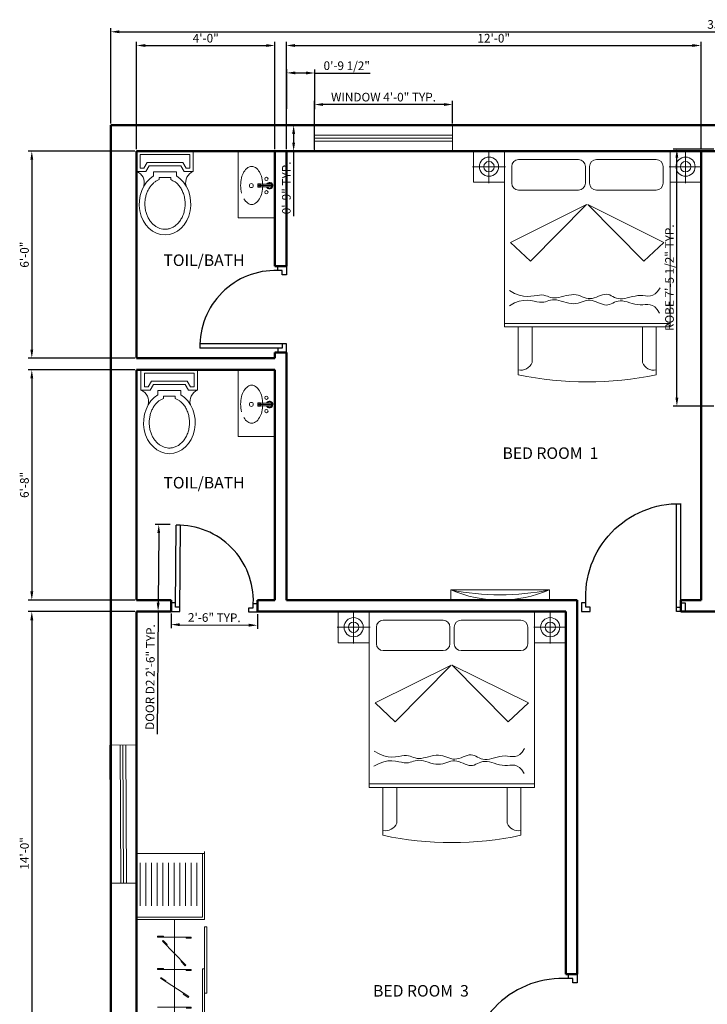
# Model space of a CAD drawing. Units: inches. Extents: x 108 to 1546, y -229 to 513.
# Tile 5 of 11: x 591 to 830, y 171 to 513. Entities that reach past the tile are written whole.
import ezdxf

# ---------------------------------------------------------------- set-up
doc = ezdxf.new("R2010")
doc.units = ezdxf.units.IN
for name, color, linetype, lineweight in [('A-ANNO-DIMS', 2, 'Continuous', 18), ('A-AREA-IDEN', 4, 'Continuous', 18), ('A-FLOR-FIXT', 9, 'Continuous', 18), ('A-FURN', 8, 'Continuous', 13), ('door', 1, 'Continuous', 25), ('tv', 2, 'Continuous', 13), ('wall', 7, 'Continuous', 50), ('WINDOW', 212, 'Continuous', 18)]:
    doc.layers.add(name, color=color, linetype=linetype, lineweight=lineweight)
doc.styles.get("Standard").update_dxf_attribs({"font": 'arial.ttf'})
doc.dimstyles.new('ISO-25', dxfattribs={"dimtxt": 3, "dimasz": 3, "dimexe": 1.25, "dimexo": 0.625, "dimtad": 1, "dimdec": 1, "dimlunit": 3, "dimtxsty": 'Standard', "dimcen": 2.5, "dimadec": 0, "dimazin": 0, "dimtfac": 1, "dimtdec": 1, "dimtmove": 0, "dimatfit": 3, "dimfxl": 1, "dimarcsym": 0})

# ---------------------------------------------------------------- blocks, each defined once
blk = doc.blocks.new('A$C4F543DC7')
for p, q in [((0.013, 3.35, -0.169), (3.313, 3.35, -0.169)), ((0.463, 3.35, -0.169), (0.013, 3.35, -0.169)), ((0.013, 2.896, -0.169), (0.013, 3.35, -0.169)), ((0.013, 3.35, -0.169), (0.013, 2.896, -0.169)), ((0.238, 3.123, -0.439), (0.238, 3.361, -0.439)), ((0.463, 3.35, -0.169), (0.463, 0.8, -0.169)), ((2.863, 3.35, -0.169), (0.463, 3.35, -0.169)), ((0.463, 2.896, -0.169), (0.463, 3.35, -0.169)), ((2.863, 0.8, -0.169), (2.863, 3.35, -0.169)), ((2.863, 3.35, -0.169), (3.313, 3.35, -0.169)), ((2.863, 2.896, -0.169), (2.863, 3.35, -0.169)), ((3.089, 3.123, -0.439), (3.089, 3.361, -0.439)), ((3.313, 3.35, -0.169), (3.313, 2.896, -0.169)), ((3.313, 3.35, -0.169), (3.313, 2.896, -0.169)), ((1.535, 3.226, -0.169), (0.668, 3.226, -0.169)), ((2.664, 3.226, -0.169), (1.797, 3.226, -0.169)), ((0.238, 3.123, -0.439), (0, 3.123, -0.439)), ((0.238, 3.123, -0.439), (0.476, 3.123, -0.439)), ((0.238, 3.123, -0.439), (0.238, 2.885, -0.439)), ((0.568, 3.126, -0.169), (0.568, 2.884, -0.169)), ((1.635, 2.884, -0.169), (1.635, 3.126, -0.169)), ((1.697, 3.126, -0.169), (1.697, 2.884, -0.169)), ((2.764, 2.884, -0.169), (2.764, 3.126, -0.169)), ((3.089, 3.123, -0.439), (2.851, 3.123, -0.439)), ((3.089, 3.123, -0.439), (3.089, 2.885, -0.439)), ((3.089, 3.123, -0.439), (3.327, 3.123, -0.439)), ((0.463, 2.896, -0.169), (0.013, 2.896, -0.169)), ((0.013, 2.896, -0.169), (0.463, 2.896, -0.169)), ((0.463, 0.8, -0.169), (0.463, 2.896, -0.169)), ((2.863, 2.896, -0.169), (2.863, 0.8, -0.169)), ((3.313, 2.896, -0.169), (2.863, 2.896, -0.169)), ((3.313, 2.896, -0.169), (2.863, 2.896, -0.169)), ((0.668, 2.784, -0.169), (1.535, 2.784, -0.169)), ((1.797, 2.784, -0.169), (2.664, 2.784, -0.169)), ((1.653, 2.573, -0.169), (0.55, 2.025, -0.169)), ((0.841, 1.752, -0.169), (1.653, 2.573, -0.169)), ((2.481, 1.752, -0.169), (1.669, 2.573, -0.169)), ((1.669, 2.573, -0.169), (2.772, 2.025, -0.169)), ((0.55, 2.025, -0.169), (0.841, 1.752, -0.169)), ((2.772, 2.025, -0.169), (2.481, 1.752, -0.169)), ((0.537, 1.327, -0.169), (0.609, 1.284, -0.169)), ((2.648, 1.277, -0.169), (2.683, 1.312, -0.169)), ((2.683, 1.312, -0.169), (2.718, 1.364, -0.169)), ((0.533, 1.105, -0.169), (0.607, 1.146, -0.169)), ((0.607, 1.146, -0.169), (0.674, 1.171, -0.169)), ((0.609, 1.284, -0.169), (0.676, 1.257, -0.169)), ((0.674, 1.171, -0.169), (0.736, 1.183, -0.169)), ((0.676, 1.257, -0.169), (0.737, 1.243, -0.169)), ((0.736, 1.183, -0.169), (0.793, 1.185, -0.169)), ((0.737, 1.243, -0.169), (0.794, 1.239, -0.169)), ((0.793, 1.185, -0.169), (0.845, 1.18, -0.169)), ((0.794, 1.239, -0.169), (0.846, 1.242, -0.169)), ((0.845, 1.18, -0.169), (0.891, 1.172, -0.169)), ((0.846, 1.242, -0.169), (0.893, 1.249, -0.169)), ((0.891, 1.172, -0.169), (0.933, 1.163, -0.169)), ((0.893, 1.249, -0.169), (0.935, 1.256, -0.169)), ((0.933, 1.163, -0.169), (0.97, 1.156, -0.169)), ((0.935, 1.256, -0.169), (0.972, 1.261, -0.169)), ((0.97, 1.156, -0.169), (1.003, 1.155, -0.169)), ((0.972, 1.261, -0.169), (1.004, 1.262, -0.169)), ((1.003, 1.155, -0.169), (1.032, 1.158, -0.169)), ((1.004, 1.262, -0.169), (1.033, 1.258, -0.169)), ((1.032, 1.158, -0.169), (1.058, 1.164, -0.169)), ((1.033, 1.258, -0.169), (1.06, 1.251, -0.169)), ((1.058, 1.164, -0.169), (1.083, 1.172, -0.169)), ((1.06, 1.251, -0.169), (1.084, 1.242, -0.169)), ((1.083, 1.172, -0.169), (1.107, 1.18, -0.169)), ((1.084, 1.242, -0.169), (1.108, 1.234, -0.169)), ((1.107, 1.18, -0.169), (1.132, 1.187, -0.169)), ((1.108, 1.234, -0.169), (1.132, 1.226, -0.169)), ((1.132, 1.226, -0.169), (1.158, 1.22, -0.169)), ((1.132, 1.187, -0.169), (1.157, 1.192, -0.169)), ((1.157, 1.192, -0.169), (1.185, 1.193, -0.169)), ((1.158, 1.22, -0.169), (1.185, 1.218, -0.169)), ((1.185, 1.218, -0.169), (1.216, 1.22, -0.169)), ((1.185, 1.193, -0.169), (1.216, 1.19, -0.169)), ((1.216, 1.22, -0.169), (1.25, 1.226, -0.169)), ((1.216, 1.19, -0.169), (1.249, 1.183, -0.169)), ((1.249, 1.183, -0.169), (1.284, 1.173, -0.169)), ((1.25, 1.226, -0.169), (1.285, 1.235, -0.169)), ((1.284, 1.173, -0.169), (1.321, 1.163, -0.169)), ((1.285, 1.235, -0.169), (1.322, 1.244, -0.169)), ((1.321, 1.163, -0.169), (1.358, 1.152, -0.169)), ((1.322, 1.244, -0.169), (1.359, 1.253, -0.169)), ((1.358, 1.152, -0.169), (1.394, 1.143, -0.169)), ((1.359, 1.253, -0.169), (1.396, 1.261, -0.169)), ((1.394, 1.143, -0.169), (1.431, 1.137, -0.169)), ((1.396, 1.261, -0.169), (1.433, 1.266, -0.169)), ((1.433, 1.266, -0.169), (1.468, 1.268, -0.169)), ((1.468, 1.268, -0.169), (1.501, 1.264, -0.169)), ((1.499, 1.137, -0.169), (1.531, 1.143, -0.169)), ((1.501, 1.264, -0.169), (1.532, 1.257, -0.169)), ((1.531, 1.143, -0.169), (1.561, 1.152, -0.169)), ((1.532, 1.257, -0.169), (1.562, 1.247, -0.169)), ((1.561, 1.152, -0.169), (1.59, 1.162, -0.169)), ((1.562, 1.247, -0.169), (1.591, 1.237, -0.169)), ((1.59, 1.162, -0.169), (1.619, 1.172, -0.169)), ((1.591, 1.237, -0.169), (1.62, 1.226, -0.169)), ((1.619, 1.172, -0.169), (1.648, 1.18, -0.169)), ((1.62, 1.226, -0.169), (1.648, 1.217, -0.169)), ((1.648, 1.217, -0.169), (1.676, 1.211, -0.169)), ((1.648, 1.18, -0.169), (1.676, 1.185, -0.169)), ((1.676, 1.211, -0.169), (1.705, 1.209, -0.169)), ((1.676, 1.185, -0.169), (1.705, 1.186, -0.169)), ((1.705, 1.209, -0.169), (1.735, 1.212, -0.169)), ((1.705, 1.186, -0.169), (1.734, 1.182, -0.169)), ((1.734, 1.182, -0.169), (1.764, 1.173, -0.169)), ((1.735, 1.212, -0.169), (1.765, 1.22, -0.169)), ((1.764, 1.173, -0.169), (1.794, 1.162, -0.169)), ((1.765, 1.22, -0.169), (1.795, 1.23, -0.169)), ((1.794, 1.162, -0.169), (1.824, 1.149, -0.169)), ((1.795, 1.23, -0.169), (1.826, 1.242, -0.169)), ((1.824, 1.149, -0.169), (1.854, 1.137, -0.169)), ((1.826, 1.242, -0.169), (1.856, 1.253, -0.169)), ((1.856, 1.253, -0.169), (1.885, 1.263, -0.169)), ((1.885, 1.263, -0.169), (1.913, 1.27, -0.169)), ((1.913, 1.27, -0.169), (1.94, 1.272, -0.169)), ((1.94, 1.272, -0.169), (1.965, 1.269, -0.169)), ((1.965, 1.269, -0.169), (1.989, 1.262, -0.169)), ((1.989, 1.262, -0.169), (2.012, 1.251, -0.169)), ((2.011, 1.134, -0.169), (2.034, 1.145, -0.169)), ((2.012, 1.251, -0.169), (2.036, 1.239, -0.169)), ((2.034, 1.145, -0.169), (2.059, 1.157, -0.169)), ((2.036, 1.239, -0.169), (2.06, 1.227, -0.169)), ((2.059, 1.157, -0.169), (2.084, 1.167, -0.169)), ((2.06, 1.227, -0.169), (2.085, 1.216, -0.169)), ((2.084, 1.167, -0.169), (2.111, 1.174, -0.169)), ((2.085, 1.216, -0.169), (2.112, 1.208, -0.169)), ((2.111, 1.174, -0.169), (2.14, 1.177, -0.169)), ((2.112, 1.208, -0.169), (2.141, 1.204, -0.169)), ((2.14, 1.177, -0.169), (2.172, 1.175, -0.169)), ((2.141, 1.204, -0.169), (2.172, 1.205, -0.169)), ((2.172, 1.205, -0.169), (2.206, 1.21, -0.169)), ((2.172, 1.175, -0.169), (2.206, 1.169, -0.169)), ((2.206, 1.21, -0.169), (2.242, 1.218, -0.169)), ((2.206, 1.169, -0.169), (2.241, 1.16, -0.169)), ((2.241, 1.16, -0.169), (2.278, 1.149, -0.169)), ((2.242, 1.218, -0.169), (2.279, 1.228, -0.169)), ((2.278, 1.149, -0.169), (2.316, 1.138, -0.169)), ((2.279, 1.228, -0.169), (2.317, 1.238, -0.169)), ((2.317, 1.238, -0.169), (2.356, 1.246, -0.169)), ((2.356, 1.246, -0.169), (2.394, 1.253, -0.169)), ((2.394, 1.253, -0.169), (2.433, 1.255, -0.169)), ((2.433, 1.255, -0.169), (2.47, 1.253, -0.169)), ((2.47, 1.253, -0.169), (2.506, 1.249, -0.169)), ((2.506, 1.249, -0.169), (2.542, 1.246, -0.169)), ((2.542, 1.246, -0.169), (2.578, 1.248, -0.169)), ((2.578, 1.248, -0.169), (2.613, 1.257, -0.169)), ((2.613, 1.257, -0.169), (2.648, 1.277, -0.169)), ((1.431, 1.137, -0.169), (1.466, 1.135, -0.169)), ((1.466, 1.135, -0.169), (1.499, 1.137, -0.169)), ((1.854, 1.137, -0.169), (1.883, 1.126, -0.169)), ((1.883, 1.126, -0.169), (1.911, 1.119, -0.169)), ((1.911, 1.119, -0.169), (1.937, 1.115, -0.169)), ((1.937, 1.115, -0.169), (1.963, 1.118, -0.169)), ((1.963, 1.118, -0.169), (1.987, 1.124, -0.169)), ((1.987, 1.124, -0.169), (2.011, 1.134, -0.169)), ((2.316, 1.138, -0.169), (2.354, 1.128, -0.169)), ((2.354, 1.128, -0.169), (2.392, 1.121, -0.169)), ((2.392, 1.121, -0.169), (2.43, 1.117, -0.169)), ((2.43, 1.117, -0.169), (2.468, 1.118, -0.169)), ((2.468, 1.118, -0.169), (2.504, 1.121, -0.169)), ((2.504, 1.121, -0.169), (2.54, 1.123, -0.169)), ((2.54, 1.123, -0.169), (2.576, 1.12, -0.169)), ((2.576, 1.12, -0.169), (2.611, 1.109, -0.169)), ((2.611, 1.109, -0.169), (2.645, 1.088, -0.169)), ((2.645, 1.088, -0.169), (2.679, 1.052, -0.169)), ((2.679, 1.052, -0.169), (2.712, 0.999, -0.169)), ((0.463, 0.85, -0.169), (2.863, 0.85, -0.169)), ((0.463, 0.8, -0.169), (2.863, 0.8, -0.169)), ((0.663, 0.8, -0.169), (0.463, 0.8, -0.169)), ((0.663, 0.8, -0.169), (2.663, 0.8, -0.169)), ((0.663, 0.104, -0.169), (0.663, 0.8, -0.169)), ((0.663, 0.104, -0.169), (0.663, 0.8, -0.169)), ((0.863, 0.281, -0.169), (0.863, 0.8, -0.169)), ((2.463, 0.8, -0.169), (2.463, 0.281, -0.169)), ((2.863, 0.8, -0.169), (2.663, 0.8, -0.169)), ((2.663, 0.8, -0.169), (2.663, 0.104, -0.169)), ((2.663, 0.8, -0.169), (2.663, 0.104, -0.169))]:
    blk.add_line(p, q)
for centre, radius in [((0.238, 3.123, -0.439), 0.139), ((0.238, 3.123, -0.439), 0.075), ((3.089, 3.123, -0.439), 0.139), ((3.089, 3.123, -0.439), 0.075)]:
    blk.add_circle(centre, radius)
for centre, radius, start, end in [((0.668, 3.126, -0.169), 0.1, 90, 180), ((1.535, 3.126, -0.169), 0.1, 0, 90), ((1.797, 3.126, -0.169), 0.1, 90, 180), ((2.664, 3.126, -0.169), 0.1, 0, 90), ((0.668, 2.884, -0.169), 0.1, 180, 270), ((1.535, 2.884, -0.169), 0.1, 270, 0), ((1.797, 2.884, -0.169), 0.1, 180, 270), ((2.664, 2.884, -0.169), 0.1, 270, 0), ((0.699, 0.347, -0.169), 0.177, 258.2616, 338.032), ((2.627, 0.347, -0.169), 0.177, 201.968, 281.7384), ((1.663, 4.86, -0.169), 4.86, 258.1252, 281.8748), ((1.663, 4.86, -0.169), 4.86, 258.1252, 281.8748)]:
    blk.add_arc(centre, radius, start, end)
blk = doc.blocks.new('A$C7C8779AE')
for p, q in [((0, 0.7405), (0, 0.5605)), ((0.5, 0.7405), (0, 0.7405)), ((0.47, 0.7105), (0.03, 0.7105)), ((0.03, 0.7105), (0.03, 0.5905)), ((0.47, 0.5905), (0.47, 0.7105)), ((0.5, 0.5605), (0.5, 0.7405)), ((0.093, 0.6405), (0.063, 0.5905)), ((0.11, 0.6105), (0.08, 0.5605)), ((0.093, 0.6405), (0.407, 0.6405)), ((0.11, 0.6105), (0.39, 0.6105)), ((0.42, 0.5605), (0.39, 0.6105)), ((0.437, 0.5905), (0.407, 0.6405)), ((0, 0.5605), (0.08, 0.5605)), ((0.03, 0.5905), (0.063, 0.5905)), ((0.1497, 0.557), (0.1497, 0.5203)), ((0.1497, 0.557), (0.3514, 0.557)), ((0.3514, 0.557), (0.3514, 0.5203)), ((0.42, 0.5605), (0.5, 0.5605)), ((0.437, 0.5905), (0.47, 0.5905)), ((0.1997, 0.507), (0.1997, 0.4879)), ((0.1997, 0.507), (0.3014, 0.507)), ((0.3014, 0.507), (0.3014, 0.4879))]:
    blk.add_line(p, q)
for centre, start, end in [((-0.0386, 0.4613), 344.64203, 68.73386), ((0.5386, 0.4613), 111.26614, 195.35797)]:
    blk.add_arc(centre, 0.1064, start, end)
blk.add_ellipse((0.2506, 0.2744), major_axis=(0, 0.2744), ratio=0.828948, start_param=0.459479, end_param=5.823706)
blk.add_open_spline([(0.1997, 0.4879), (0.1697, 0.474), (0.1642, 0.4702), (0.1512, 0.4602), (0.1438, 0.4535), (0.1298, 0.4388), (0.1233, 0.4306), (0.1111, 0.4131), (0.1055, 0.4037), (0.0956, 0.3838), (0.0912, 0.3733), (0.0838, 0.3516), (0.0808, 0.3403), (0.0762, 0.3172), (0.0746, 0.3055), (0.073, 0.2817), (0.0729, 0.2698), (0.0743, 0.246), (0.0758, 0.2342), (0.0801, 0.2111), (0.0831, 0.1998), (0.0903, 0.1779), (0.0945, 0.1673), (0.1043, 0.1473), (0.1098, 0.1378), (0.1218, 0.12), (0.1283, 0.1118), (0.1421, 0.0968), (0.1494, 0.09), (0.1646, 0.078), (0.1725, 0.0728), (0.1887, 0.064), (0.1969, 0.0603), (0.2137, 0.0547), (0.2222, 0.0527), (0.2392, 0.0502), (0.2478, 0.0498), (0.2664, 0.0505), (0.2764, 0.052), (0.2963, 0.0573), (0.3061, 0.061), (0.3253, 0.0707), (0.3346, 0.0766), (0.3525, 0.0906), (0.3611, 0.0987), (0.3771, 0.1169), (0.3845, 0.127), (0.3978, 0.1488), (0.4037, 0.1605), (0.4137, 0.1853), (0.4178, 0.1983), (0.424, 0.2251), (0.4261, 0.2389), (0.4282, 0.2668), (0.4283, 0.2809), (0.4262, 0.3088), (0.4241, 0.3226), (0.418, 0.3495), (0.414, 0.3625), (0.404, 0.3873), (0.3982, 0.3991), (0.385, 0.421), (0.3776, 0.4311), (0.3617, 0.4494), (0.3531, 0.4575), (0.3382, 0.4693), (0.3321, 0.4736), (0.3014, 0.4879)], degree=3, knots=[0.459479, 0.459479, 0.459479, 0.459479, 0.567422, 0.567422, 0.720865, 0.720865, 0.874307, 0.874307, 1.02775, 1.02775, 1.181192, 1.181192, 1.334635, 1.334635, 1.488077, 1.488077, 1.64152, 1.64152, 1.794963, 1.794963, 1.948405, 1.948405, 2.101848, 2.101848, 2.25529, 2.25529, 2.408733, 2.408733, 2.562175, 2.562175, 2.715618, 2.715618, 2.86906, 2.86906, 3.022503, 3.022503, 3.175946, 3.175946, 3.356457, 3.356457, 3.536968, 3.536968, 3.717479, 3.717479, 3.89799, 3.89799, 4.078501, 4.078501, 4.259012, 4.259012, 4.439523, 4.439523, 4.620035, 4.620035, 4.800546, 4.800546, 4.981057, 4.981057, 5.161568, 5.161568, 5.342079, 5.342079, 5.52259, 5.52259, 5.703101, 5.703101, 5.823706, 5.823706, 5.823706, 5.823706])
blk = doc.blocks.new('A$C34930FF8')
for p, q in [((600, 1669.3), (600, 2269.3)), ((580, 1690.9), (580, 2252.4)), ((30, 1790.9), (30, 2169.3)), ((80, 1790.9), (80, 2169.3)), ((130, 1790.9), (130, 2169.3)), ((180, 1790.9), (180, 2169.3)), ((230, 1790.9), (230, 2169.3)), ((280, 1790.9), (280, 2169.3)), ((330, 1790.9), (330, 2169.3)), ((380, 1790.9), (380, 2169.3)), ((430, 1790.9), (430, 2169.3)), ((480, 1790.9), (480, 2169.3)), ((530, 1790.9), (530, 2169.3)), ((580, 1690.9), (0, 1690.9)), ((600, 1669.3), (0, 1669.3)), ((335.4, 1666.1), (335.4, 603.1)), ((600, 1603.3), (620, 1603.3)), ((600, 1018.7), (600, 1603.3)), ((620, 1603.3), (620, 1018.7)), ((237.7, 1521.5), (185.4, 1521.5)), ((482.5, 1513), (185.4, 1513)), ((434.8, 1266.1), (227.4, 1478.9)), ((269.7, 1447.7), (233.2, 1485.2)), ((436.7, 1504.4), (482.5, 1504.4)), ((237.7, 1237.7), (185.4, 1237.7)), ((482.5, 1228.2), (185.4, 1228.2)), ((428.7, 1260.1), (392.1, 1297.6)), ((436.7, 1219.7), (482.5, 1219.7)), ((600, 1233.4), (580, 1233.4)), ((580, 1233.4), (580, 648.7)), ((600, 648.7), (600, 1233.4)), ((459.3, 989.3), (209.5, 1150.1)), ((258.1, 1129), (214.1, 1157.3)), ((454.7, 982.1), (410.6, 1010.5)), ((620, 1018.7), (600, 1018.7)), ((482.5, 894.9), (185.4, 894.9)), ((436.7, 886.3), (482.5, 886.3)), ((237.7, 783.9), (185.4, 783.9)), ((482.5, 775.3), (185.4, 775.3)), ((436.7, 766.8), (482.5, 766.8)), ((580, 648.7), (600, 648.7)), ((600, 600), (0, 600)), ((580, 578.3), (0, 578.3)), ((580, 578.3), (580, 16.8)), ((600, 600), (600, 0)), ((30, 478.3), (30, 100)), ((80, 478.3), (80, 100)), ((130, 478.3), (130, 100)), ((180, 478.3), (180, 100)), ((230, 478.3), (230, 100)), ((280, 478.3), (280, 100)), ((330, 478.3), (330, 100)), ((380, 478.3), (380, 100)), ((430, 478.3), (430, 100)), ((480, 478.3), (480, 100)), ((530, 478.3), (530, 100))]:
    blk.add_line(p, q)
at = {"ltscale": 0.05}
for p, q in [((0, 2252.4), (0, 16.8)), ((600, 2252.4), (0, 2252.4)), ((185.4, 1513), (185.4, 1521.5)), ((227.1, 1479.2), (233.2, 1485.2)), ((237.7, 1513), (237.7, 1521.5)), ((436.7, 1513), (436.7, 1504.4)), ((482.5, 1513), (482.5, 1504.4)), ((263.6, 1441.7), (269.7, 1447.7)), ((398.2, 1303.6), (392.1, 1297.6)), ((185.4, 1229.1), (185.4, 1237.7)), ((237.7, 1229.1), (237.7, 1237.7)), ((434.8, 1266.1), (428.7, 1260.1)), ((436.7, 1228.2), (436.7, 1219.7)), ((482.5, 1228.2), (482.5, 1219.7)), ((209.5, 1150.1), (214.1, 1157.3)), ((253.5, 1121.8), (258.1, 1129)), ((415.3, 1017.6), (410.6, 1010.5)), ((459.3, 989.3), (454.7, 982.1)), ((482.5, 894.9), (482.5, 886.3)), ((237.7, 775.3), (237.7, 783.9)), ((436.7, 775.3), (436.7, 766.8)), ((482.5, 775.3), (482.5, 766.8)), ((600, 16.8), (0, 16.8))]:
    blk.add_line(p, q, dxfattribs=at)
blk = doc.blocks.new('*D23')
at = {"layer": 'A-ANNO-DIMS', "color": 0, "lineweight": -2, "transparency": 16777216}
for p, q in [((623, 477.09), (623, 510.15)), ((1043, 477.09), (1043, 510.15)), ((626, 508.9), (1040, 508.9))]:
    blk.add_line(p, q, dxfattribs=at)
at = {"layer": 'A-ANNO-DIMS', "color": 0, "transparency": 16777216}
for points in [[(626, 509.4), (626, 508.4), (623, 508.9)], [(1040, 509.4), (1040, 508.4), (1043, 508.9)]]:
    blk.add_solid(points, dxfattribs=at)
at = {"layer": 'Defpoints', "color": 0, "transparency": 16777216}
for p in [(1043, 508.9), (623, 476.47), (1043, 476.47)]:
    blk.add_point(p, dxfattribs=at)
at = {"layer": 'A-ANNO-DIMS', "color": 0, "transparency": 16777216, "insert": (833, 511.06), "char_height": 3, "attachment_point": 5}
blk.add_mtext("35'", dxfattribs=at)
blk = doc.blocks.new('WINDOW-48X9')
for p, q in [((0, 9), (0, 0)), ((0, 9), (48, 9)), ((48, 9), (48, 0)), ((0, 5.5), (48, 5.5)), ((0, 4.5), (48, 4.5)), ((0, 3.5), (48, 3.5)), ((0, 0), (48, 0))]:
    blk.add_line(p, q)
blk = doc.blocks.new('DOOR-SWING-36')
for p, q in [((1.5, 1.5), (1.5, 37.5)), ((3, 1.5), (3, 37.5)), ((0, 3), (0, 0)), ((1.5, 3), (0, 3)), ((1.5, 1.5), (1.5, 3)), ((3, 1.5), (1.5, 1.5)), ((3, 0), (3, 1.5)), ((33, 0), (33, 1.5)), ((33, 1.5), (34.5, 1.5)), ((34.5, 1.5), (34.5, 3)), ((34.5, 3), (36, 3)), ((36, 3), (36, 0)), ((0, 0), (3, 0)), ((36, 0), (33, 0))]:
    blk.add_line(p, q)
blk.add_arc((2.25, 5.18), 32.32, 356.1244, 91.3295)
blk = doc.blocks.new('DOOR-SWING-30')
for p, q in [((27, 30), (30, 30)), ((27, 28.5), (27, 30)), ((28.5, 28.5), (27, 28.5)), ((28.5, 27), (28.5, 28.5)), ((30, 30), (30, 27)), ((30, 27), (28.5, 27)), ((30, 3), (0, 3)), ((28.5, 1.5), (0, 1.5)), ((28.5, 1.5), (27, 1.5)), ((27, 1.5), (27, 0)), ((30, 3), (28.5, 3)), ((28.5, 3), (28.5, 1.5)), ((30, 0), (30, 3)), ((27, 0), (30, 0))]:
    blk.add_line(p, q)
blk.add_arc((26.25, 2.25), 26.26, 88.3634, 181.6366)
blk = doc.blocks.new('TV-WALL-MOUNT')
blk.add_lwpolyline([(0, 0), (34.19, 0), (34.19, 3.56), (0, 3.56)], close=True)
for centre, radius, start, end in [((17.1, 42.8), 42.8, 246.4582, 293.5418), ((17.1, 84.72), 82.93, 258.1036, 281.8964)]:
    blk.add_arc(centre, radius, start, end)
blk = doc.blocks.new('LAVATORY-COMPACT')
for p, q in [((12.75, 23.17), (0, 23.17)), ((0, 23.17), (0, 0)), ((0, 23.17), (0, 0)), ((12.75, 23.17), (12.75, 0)), ((7.76, 11.74), (6.84, 11.74)), ((6.84, 11.74), (6.84, 10.58)), ((7.76, 10.58), (6.84, 10.58)), ((11.59, 11.62), (6.95, 11.62)), ((6.95, 11.62), (6.95, 10.7)), ((11.59, 11.16), (6.95, 11.16)), ((11.59, 10.7), (6.95, 10.7)), ((7.53, 11.62), (7.53, 10.7)), ((7.76, 11.74), (7.76, 10.58)), ((11.59, 11.62), (11.59, 10.7)), ((12.75, 0), (0, 0))]:
    blk.add_line(p, q)
for centre, radius in [((9.83, 13.48), 0.579), ((4.59, 11.16), 0.69), ((9.83, 8.84), 0.579)]:
    blk.add_circle(centre, radius)
for centre, radius, start, end in [((6.18, 13.48), 4.82, 125.5822, 149.9314), ((4.71, 15.53), 2.3, 90, 125.5822), ((4.71, 15.53), 2.3, 54.4178, 90), ((3.24, 13.48), 4.82, 30.0686, 54.4178), ((12.25, 11.22), 11.37, 166.5147, 180), ((8.53, 12.12), 7.54, 149.9314, 166.5147), ((0.89, 12.12), 7.54, 13.4853, 30.0686), ((-2.84, 11.22), 11.37, 360, 13.4853), ((12.25, 11.22), 11.37, 180, 193.4853), ((-2.84, 11.22), 11.37, 346.5147, 0), ((10.9, 11.12), 1.15, 201.7425, 154.2331), ((10.9, 11.12), 0.92, 207.632, 147.0256), ((0.89, 10.33), 7.54, 329.9314, 346.5147), ((6.18, 8.97), 4.82, 210.0686, 234.4178), ((4.71, 6.91), 2.3, 234.4178, 270), ((4.71, 6.91), 2.3, 270, 305.5822), ((3.24, 8.97), 4.82, 305.5822, 329.9314)]:
    blk.add_arc(centre, radius, start, end)
blk = doc.blocks.new('*D36')
at = {"layer": 'A-ANNO-DIMS', "color": 0, "lineweight": -2, "transparency": 16777216}
for p, q in [((693.73, 477.05), (693.73, 484.88)), ((738.73, 483.63), (696.73, 483.63)), ((741.73, 477.05), (741.73, 484.88))]:
    blk.add_line(p, q, dxfattribs=at)
at = {"layer": 'A-ANNO-DIMS', "color": 0, "transparency": 16777216}
for points in [[(696.73, 484.13), (696.73, 483.13), (693.73, 483.63)], [(738.73, 484.13), (738.73, 483.13), (741.73, 483.63)]]:
    blk.add_solid(points, dxfattribs=at)
at = {"layer": 'Defpoints', "color": 0, "transparency": 16777216}
for p in [(693.73, 483.63), (693.73, 476.43), (741.73, 476.43)]:
    blk.add_point(p, dxfattribs=at)
at = {"layer": 'A-ANNO-DIMS', "color": 0, "transparency": 16777216, "insert": (717.73, 485.81), "char_height": 3, "attachment_point": 5}
blk.add_mtext('WINDOW 4\'-0" TYP.', dxfattribs=at)
blk = doc.blocks.new('*D37')
at = {"layer": 'A-ANNO-DIMS', "color": 0, "lineweight": -2, "transparency": 16777216}
for p, q in [((693.11, 476.43), (685.28, 476.43)), ((686.53, 473.43), (686.53, 470.43)), ((693.11, 467.43), (685.28, 467.43)), ((686.53, 467.43), (686.53, 444.89))]:
    blk.add_line(p, q, dxfattribs=at)
at = {"layer": 'A-ANNO-DIMS', "color": 0, "transparency": 16777216}
for points in [[(686.03, 473.43), (687.03, 473.43), (686.53, 476.43)], [(686.03, 470.43), (687.03, 470.43), (686.53, 467.43)]]:
    blk.add_solid(points, dxfattribs=at)
at = {"layer": 'Defpoints', "color": 0, "transparency": 16777216}
for p in [(693.73, 476.43), (686.53, 467.43), (693.73, 467.43)]:
    blk.add_point(p, dxfattribs=at)
at = {"layer": 'A-ANNO-DIMS', "color": 0, "transparency": 16777216, "insert": (684.38, 454.66), "char_height": 3, "attachment_point": 5, "rotation": 90}
blk.add_mtext('0\'-9" TYP.', dxfattribs=at)
blk = doc.blocks.new('*D44')
at = {"layer": 'A-ANNO-DIMS', "color": 0, "lineweight": -2, "transparency": 16777216}
for p, q in [((832.37, 468.13), (818.34, 468.13)), ((819.59, 381.79), (819.59, 465.13)), ((832.37, 378.79), (818.34, 378.79))]:
    blk.add_line(p, q, dxfattribs=at)
at = {"layer": 'A-ANNO-DIMS', "color": 0, "transparency": 16777216}
for points in [[(819.09, 465.13), (820.09, 465.13), (819.59, 468.13)], [(819.09, 381.79), (820.09, 381.79), (819.59, 378.79)]]:
    blk.add_solid(points, dxfattribs=at)
at = {"layer": 'Defpoints', "color": 0, "transparency": 16777216}
for p in [(819.59, 468.13), (833, 468.13), (833, 378.79)]:
    blk.add_point(p, dxfattribs=at)
at = {"layer": 'A-ANNO-DIMS', "color": 0, "transparency": 16777216, "insert": (817.42, 423.46), "char_height": 3, "attachment_point": 5, "rotation": 90}
blk.add_mtext('ROBE 7\'-5 1/2" TYP.', dxfattribs=at)
blk = doc.blocks.new('*D50')
at = {"layer": 'A-ANNO-DIMS', "color": 0, "lineweight": -2, "transparency": 16777216}
for p, q in [((643.61, 337.7), (638.45, 337.74)), ((639.68, 334.73), (639.49, 310.52)), ((643.37, 307.49), (638.21, 307.53)), ((639.46, 307.52), (639.13, 264.88))]:
    blk.add_line(p, q, dxfattribs=at)
at = {"layer": 'A-ANNO-DIMS', "color": 0, "transparency": 16777216}
for points in [[(639.18, 334.73), (640.18, 334.72), (639.7, 337.73)], [(638.99, 310.53), (639.99, 310.52), (639.46, 307.52)]]:
    blk.add_solid(points, dxfattribs=at)
at = {"layer": 'Defpoints', "color": 0, "transparency": 16777216}
for p in [(644.23, 337.69), (639.46, 307.52), (644, 307.49)]:
    blk.add_point(p, dxfattribs=at)
at = {"layer": 'A-ANNO-DIMS', "color": 0, "transparency": 16777216, "insert": (637.11, 284.72), "char_height": 3, "attachment_point": 5, "rotation": 89.5521}
blk.add_mtext('DOOR D2 2\'-6" TYP.', dxfattribs=at)
blk = doc.blocks.new('*D51')
at = {"layer": 'A-ANNO-DIMS', "color": 0, "lineweight": -2, "transparency": 16777216}
for p, q in [((643.99, 306.86), (643.95, 301.71)), ((673.99, 306.63), (673.95, 301.47)), ((646.96, 302.93), (670.96, 302.75))]:
    blk.add_line(p, q, dxfattribs=at)
at = {"layer": 'A-ANNO-DIMS', "color": 0, "transparency": 16777216}
for points in [[(646.96, 303.43), (646.96, 302.43), (643.96, 302.96)], [(670.96, 303.25), (670.96, 302.25), (673.96, 302.72)]]:
    blk.add_solid(points, dxfattribs=at)
at = {"layer": 'Defpoints', "color": 0, "transparency": 16777216}
for p in [(644, 307.49), (673.99, 307.25), (673.96, 302.72)]:
    blk.add_point(p, dxfattribs=at)
at = {"layer": 'A-ANNO-DIMS', "color": 0, "transparency": 16777216, "insert": (658.98, 305), "char_height": 3, "attachment_point": 5, "rotation": 359.5521}
blk.add_mtext('2\'-6" TYP.', dxfattribs=at)
blk = doc.blocks.new('*D83')
at = {"layer": 'A-ANNO-DIMS', "color": 0, "lineweight": -2, "transparency": 16777216}
for p, q in [((632, 468.09), (632, 505.38)), ((635, 504.13), (677, 504.13)), ((680, 468.09), (680, 505.38))]:
    blk.add_line(p, q, dxfattribs=at)
at = {"layer": 'A-ANNO-DIMS', "color": 0, "transparency": 16777216}
for points in [[(635, 504.63), (635, 503.63), (632, 504.13)], [(677, 504.63), (677, 503.63), (680, 504.13)]]:
    blk.add_solid(points, dxfattribs=at)
at = {"layer": 'Defpoints', "color": 0, "transparency": 16777216}
for p in [(680, 504.13), (632, 467.47), (680, 467.47)]:
    blk.add_point(p, dxfattribs=at)
at = {"layer": 'A-ANNO-DIMS', "color": 0, "transparency": 16777216, "insert": (656, 506.28), "char_height": 3, "attachment_point": 5}
blk.add_mtext('4\'-0"', dxfattribs=at)
blk = doc.blocks.new('*D84')
at = {"layer": 'A-ANNO-DIMS', "color": 0, "lineweight": -2, "transparency": 16777216}
for p, q in [((684, 468.09), (684, 505.38)), ((687, 504.13), (825, 504.13)), ((828, 468.09), (828, 505.38))]:
    blk.add_line(p, q, dxfattribs=at)
at = {"layer": 'A-ANNO-DIMS', "color": 0, "transparency": 16777216}
for points in [[(687, 504.63), (687, 503.63), (684, 504.13)], [(825, 504.63), (825, 503.63), (828, 504.13)]]:
    blk.add_solid(points, dxfattribs=at)
at = {"layer": 'Defpoints', "color": 0, "transparency": 16777216}
for p in [(828, 504.13), (684, 467.47), (828, 467.47)]:
    blk.add_point(p, dxfattribs=at)
at = {"layer": 'A-ANNO-DIMS', "color": 0, "transparency": 16777216, "insert": (756, 506.28), "char_height": 3, "attachment_point": 5}
blk.add_mtext('12\'-0"', dxfattribs=at)
blk = doc.blocks.new('*D91')
at = {"layer": 'A-ANNO-DIMS', "color": 0, "lineweight": -2, "transparency": 16777216}
for p, q in [((631.37, 467.47), (594.36, 467.47)), ((595.61, 464.47), (595.61, 398.47)), ((631.37, 395.47), (594.36, 395.47))]:
    blk.add_line(p, q, dxfattribs=at)
at = {"layer": 'A-ANNO-DIMS', "color": 0, "transparency": 16777216}
for points in [[(595.11, 464.47), (596.11, 464.47), (595.61, 467.47)], [(595.11, 398.47), (596.11, 398.47), (595.61, 395.47)]]:
    blk.add_solid(points, dxfattribs=at)
at = {"layer": 'Defpoints', "color": 0, "transparency": 16777216}
for p in [(632, 467.47), (595.61, 395.47), (632, 395.47)]:
    blk.add_point(p, dxfattribs=at)
at = {"layer": 'A-ANNO-DIMS', "color": 0, "transparency": 16777216, "insert": (593.45, 431.47), "char_height": 3, "attachment_point": 5, "rotation": 90}
blk.add_mtext('6\'-0"', dxfattribs=at)
blk = doc.blocks.new('*D92')
at = {"layer": 'A-ANNO-DIMS', "color": 0, "lineweight": -2, "transparency": 16777216}
for p, q in [((631.37, 391.47), (594.36, 391.47)), ((595.61, 388.47), (595.61, 314.47)), ((631.37, 311.47), (594.36, 311.47))]:
    blk.add_line(p, q, dxfattribs=at)
at = {"layer": 'A-ANNO-DIMS', "color": 0, "transparency": 16777216}
for points in [[(595.11, 388.47), (596.11, 388.47), (595.61, 391.47)], [(595.11, 314.47), (596.11, 314.47), (595.61, 311.47)]]:
    blk.add_solid(points, dxfattribs=at)
at = {"layer": 'Defpoints', "color": 0, "transparency": 16777216}
for p in [(632, 391.47), (595.61, 311.47), (632, 311.47)]:
    blk.add_point(p, dxfattribs=at)
at = {"layer": 'A-ANNO-DIMS', "color": 0, "transparency": 16777216, "insert": (593.45, 351.47), "char_height": 3, "attachment_point": 5, "rotation": 90}
blk.add_mtext('6\'-8"', dxfattribs=at)
blk = doc.blocks.new('*D93')
at = {"layer": 'A-ANNO-DIMS', "color": 0, "lineweight": -2, "transparency": 16777216}
for p, q in [((631.37, 307.47), (594.36, 307.47)), ((595.61, 304.47), (595.61, 142.47)), ((631.37, 139.47), (594.36, 139.47))]:
    blk.add_line(p, q, dxfattribs=at)
at = {"layer": 'A-ANNO-DIMS', "color": 0, "transparency": 16777216}
for points in [[(595.11, 304.47), (596.11, 304.47), (595.61, 307.47)], [(595.11, 142.47), (596.11, 142.47), (595.61, 139.47)]]:
    blk.add_solid(points, dxfattribs=at)
at = {"layer": 'Defpoints', "color": 0, "transparency": 16777216}
for p in [(632, 307.47), (595.61, 139.47), (632, 139.47)]:
    blk.add_point(p, dxfattribs=at)
at = {"layer": 'A-ANNO-DIMS', "color": 0, "transparency": 16777216, "insert": (593.45, 223.47), "char_height": 3, "attachment_point": 5, "rotation": 90}
blk.add_mtext('14\'-0"', dxfattribs=at)
blk = doc.blocks.new('*D99')
at = {"layer": 'A-ANNO-DIMS', "color": 0, "lineweight": -2, "transparency": 16777216}
for p, q in [((684, 468.09), (684.11, 495.87)), ((687.11, 494.61), (690.85, 494.59)), ((693.74, 468.05), (693.85, 495.83)), ((693.85, 494.58), (713.06, 494.5))]:
    blk.add_line(p, q, dxfattribs=at)
at = {"layer": 'A-ANNO-DIMS', "color": 0, "transparency": 16777216}
for points in [[(687.11, 495.11), (687.11, 494.11), (684.11, 494.62)], [(690.85, 495.09), (690.85, 494.09), (693.85, 494.58)]]:
    blk.add_solid(points, dxfattribs=at)
at = {"layer": 'Defpoints', "color": 0, "transparency": 16777216}
for p in [(693.85, 494.58), (684, 467.47), (693.73, 467.43)]:
    blk.add_point(p, dxfattribs=at)
at = {"layer": 'A-ANNO-DIMS', "color": 0, "transparency": 16777216, "insert": (704.96, 496.71), "char_height": 3, "attachment_point": 5, "rotation": 359.7607}
blk.add_mtext('0\'-9 1/2"', dxfattribs=at)

msp = doc.modelspace()

# ---------------------------------------------------------------- linework, layer by layer
at = {"layer": 'wall'}
for p, q in [((1043, 476.47), (623, 476.47)), ((623, 476.47), (623, -3.53)), ((1034, 467.47), (632, 467.47)), ((632, 467.47), (632, 395.47)), ((680, 467.47), (680, 427.47)), ((684, 467.47), (684, 427.47)), ((828, 467.47), (828, 311.47)), ((680, 427.47), (684, 427.47)), ((680, 397.47), (684, 397.47)), ((680, 397.47), (680, 395.47)), ((684, 397.47), (684, 311.47)), ((680, 395.47), (632, 395.47)), ((680, 391.47), (632, 391.47)), ((632, 391.47), (632, 311.47)), ((680, 391.47), (680, 311.47)), ((644, 311.47), (632, 311.47)), ((644, 311.47), (644, 307.47)), ((680, 311.47), (674, 311.47)), ((674, 311.47), (674, 307.47)), ((785, 311.47), (684, 311.47)), ((785, 311.47), (785, 307.47)), ((828, 311.47), (821, 311.47)), ((821, 311.47), (821, 307.47)), ((632, 307.47), (632, 139.47)), ((644, 307.47), (632, 307.47)), ((781, 307.47), (674, 307.47)), ((781, 307.47), (781, 181.47)), ((785, 307.47), (785, 181.47)), ((837, 307.47), (821, 307.47)), ((781, 181.47), (785, 181.47))]:
    msp.add_line(p, q, dxfattribs=at)

# ---------------------------------------------------------------- block references
at = {"layer": 'A-FLOR-FIXT', "xscale": 39.37007874015748, "yscale": 39.37007874015748, "zscale": 39.37007874015748}
for p in [(632, 438.32), (633.51, 362.32)]:
    msp.add_blockref('A$C7C8779AE', p, dxfattribs=at)
at = {"layer": 'A-FLOR-FIXT'}
for p in [(667.25, 444.3), (667.25, 368.3)]:
    msp.add_blockref('LAVATORY-COMPACT', p, dxfattribs=at)
at = {"layer": 'A-FURN'}
for name, p, xscale, yscale, zscale in [('A$C4F543DC7', (748.66, 387.26, 4.04), 23.94379789781286, 23.94379789781286, 23.94379789781286), ('A$C4F543DC7', (701.66, 227.26, 4.04), 23.94379789781286, 23.94379789781286, 23.94379789781286), ('A$C34930FF8', (632, 134.79), 0.0393700787401575, 0.0393700787401575, 0.0393700787401575)]:
    msp.add_blockref(name, p, dxfattribs=dict(at, xscale=xscale, yscale=yscale, zscale=zscale))
at = {"layer": 'door'}
msp.add_blockref('DOOR-SWING-30', (653.99, 397.47), dxfattribs=at)
at = {"layer": 'door', "extrusion": (0, 0, -1), "zscale": -1}
msp.add_blockref('DOOR-SWING-36', (-822.5, 307.47), dxfattribs=at)
at = {"layer": 'door'}
for name, p, rotation in [('DOOR-SWING-30', (644.23, 337.49), 269.5521447183099), ('DOOR-SWING-36', (785, 145.47), 90.00000000000031)]:
    msp.add_blockref(name, p, dxfattribs=dict(at, rotation=rotation))
at = {"layer": 'tv'}
msp.add_blockref('TV-WALL-MOUNT', (741.12, 311.47), dxfattribs=at)
at = {"layer": 'WINDOW'}
for p, rotation in [((741.73, 476.43), 180), ((631.99, 213.15), 90.2799560098104)]:
    msp.add_blockref('WINDOW-48X9', p, dxfattribs=dict(at, rotation=rotation))

# ---------------------------------------------------------------- texts
at = {"layer": 'A-AREA-IDEN', "char_height": 4, "attachment_point": 1}
for s, insert in [('TOIL/BATH', (641.32, 431.54)), ('BED ROOM  1', (759.06, 364.52)), ('TOIL/BATH', (641.32, 354.24)), ('BED ROOM  3', (714.11, 177.73))]:
    msp.add_mtext_dynamic_manual_height_columns(s, width=57.4311, gutter_width=12.5, heights=[12.84], dxfattribs=dict(at, insert=insert))

# ---------------------------------------------------------------- dimensions: what is measured, and where the dimension line sits
at = {"layer": 'A-ANNO-DIMS'}
for base, p1, p2, override, picture, middle in [((1043, 508.9), (623, 476.47), (1043, 476.47), {"dimclrd": 0, "dimclre": 0, "dimclrt": 0}, '*D23', (833, 511.06)), ((680, 504.13), (632, 467.47), (680, 467.47), {"dimdec": 1, "dimlfac": 1, "dimrnd": 0, "dimzin": 1, "dimdsep": 46, "dimlunit": 4, "dimfrac": 2}, '*D83', (656, 506.28)), ((828, 504.13), (684, 467.47), (828, 467.47), {"dimdec": 1, "dimlfac": 1, "dimrnd": 0, "dimzin": 1, "dimdsep": 46, "dimlunit": 4, "dimfrac": 2}, '*D84', (756, 506.28))]:
    dim = msp.add_linear_dim(base=base, p1=p1, p2=p2, dimstyle='ISO-25', override=override, dxfattribs=at)
    dim.commit()
    dim.dimension.update_dxf_attribs({"geometry": picture, "text_midpoint": middle})
for base, p1, p2, angle, picture, middle in [((693.85, 494.58), (684, 467.47), (693.73, 467.43), 359.7607, '*D99', (704.96, 496.71)), ((595.61, 395.47), (632, 467.47), (632, 395.47), 90, '*D91', (593.45, 431.47)), ((595.61, 311.47), (632, 391.47), (632, 311.47), 90, '*D92', (593.45, 351.47)), ((595.61, 139.47), (632, 307.47), (632, 139.47), 90, '*D93', (593.45, 223.47))]:
    dim = msp.add_linear_dim(base=base, p1=p1, p2=p2, angle=angle, dimstyle='ISO-25', override={"dimdec": 1, "dimlfac": 1, "dimrnd": 0, "dimzin": 1, "dimdsep": 46, "dimlunit": 4, "dimfrac": 2}, dxfattribs=at)
    dim.commit()
    dim.dimension.update_dxf_attribs({"geometry": picture, "text_midpoint": middle})
for base, p1, p2, angle, text, picture, middle in [((693.73, 483.63), (741.73, 476.43), (693.73, 476.43), 180, 'WINDOW <> TYP.', '*D36', (717.73, 485.81)), ((686.53, 467.43), (693.73, 476.43), (693.73, 467.43), 270, '<> TYP.', '*D37', (684.38, 454.66)), ((819.59, 468.13), (833, 378.79), (833, 468.13), 90, 'ROBE <> TYP.', '*D44', (817.42, 423.46)), ((639.46, 307.52), (644.23, 337.69), (644, 307.49), 269.5521, 'DOOR D2 <> TYP.', '*D50', (637.11, 284.72)), ((673.96, 302.72), (644, 307.49), (673.99, 307.25), 359.5521, '<> TYP.', '*D51', (658.98, 305))]:
    dim = msp.add_linear_dim(base=base, p1=p1, p2=p2, angle=angle, text=text, dimstyle='ISO-25', override={"dimdec": 1, "dimlfac": 1, "dimrnd": 0, "dimzin": 1, "dimdsep": 46, "dimlunit": 4, "dimfrac": 2}, dxfattribs=at)
    dim.commit()
    dim.dimension.update_dxf_attribs({"geometry": picture, "text_midpoint": middle})

doc.saveas('drawing.dxf')
